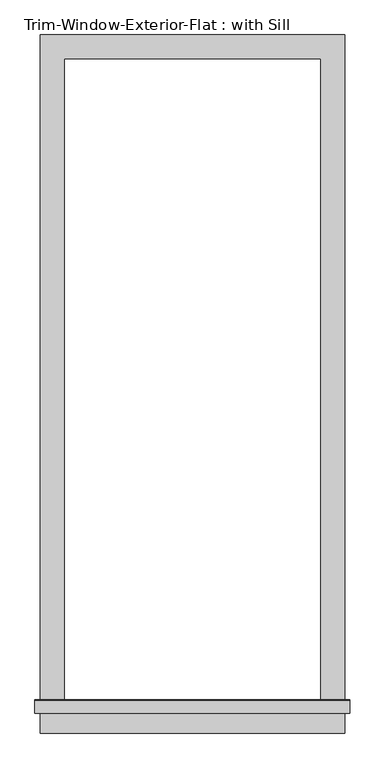
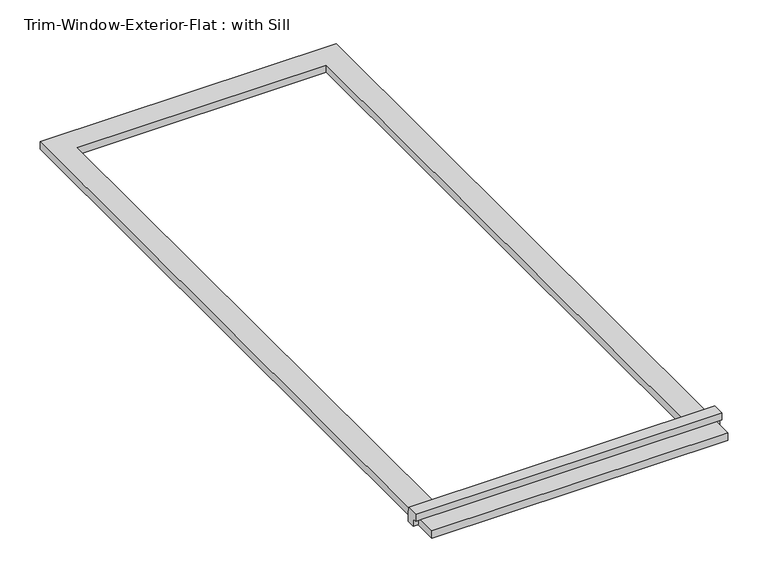
"""IFC4 building model written with IfcOpenShell, lengths in millimetres: proxy geometry, Trim-Window-Exterior-Flat : with Sill."""

from ifc_helpers import new_model, si_unit, frame, origin, origin_with_axes, place, context, project, spatial, polyline, outline, extrude, source, transform, mapped, element, save


def trim_window_exterior_flat_with_sill_4912eb0d(model_context):
    return source(origin(), model_context, "Body", "SweptSolid", [
        extrude(outline(polyline([(361.95, -1546.1823709), (361.95, -1603.3323709), (-361.95, -1603.3323709), (-361.95, -1546.1823709), (361.95, -1546.1823709)])), origin_with_axes(), (0.0, 0.0, 1.0), 19.05),
        extrude(outline(polyline([(-1555.75, 38.1), (-1526.4580645, 38.1), (-1524.0, 19.05), (-1524.0, 0.0), (-1546.1823709, 0.0), (-1546.1823709, 19.05), (-1555.75, 19.05), (-1555.75, 38.1)])), frame((-374.65, 0.0, 0.0), z_axis=(1.0, 0.0, 0.0), x_axis=(0.0, 1.0, 0.0)), (0.0, 0.0, 1.0), 749.3),
        extrude(outline(polyline([(-361.95, 57.15), (361.95, 57.15), (361.95, -1524.0), (304.8, -1524.0), (304.8, 0.0), (-304.8, 0.0), (-304.8, -1524.0), (-361.95, -1524.0), (-361.95, 57.15)])), origin_with_axes(), (0.0, 0.0, 1.0), 19.05),
    ])


if __name__ == "__main__":
    model = new_model("IFC4")
    model_context = context("Model", 3, world=origin())
    ifc_project = project(units=[si_unit("LENGTHUNIT", "METRE", prefix="MILLI")], contexts=[model_context])
    site = spatial("IfcSite", under=ifc_project)
    building = spatial("IfcBuilding", under=site)
    placement = place(None, origin())
    trim_window_exterior_flat_with_sill_shape = trim_window_exterior_flat_with_sill_4912eb0d(model_context)
    element("IfcBuildingElementProxy", 1, Name="Trim-Window-Exterior-Flat : with Sill", ObjectType="Trim-Window-Exterior-Flat : with Sill", at=placement, inside=building, context=model_context, shape_type="MappedRepresentation", body=[
        mapped(trim_window_exterior_flat_with_sill_shape, transform((0.0, 0.0, 0.0), x_axis=(1.0, 0.0, 0.0), y_axis=(0.0, 1.0, 0.0), z_axis=(0.0, 0.0, 1.0))),
    ])
    save(model, "model.ifc")

# Revit data of these elements
# Type "Trim-Window-Exterior-Flat : with Sill"
#   Trim Width = 0' - 2 1/4"
#   Trim Thickness_Picture Frame = 0' - 1 1/4"
#   Trim Thickness_with Sill = 0' - 0 3/4"
#   Sill Thickness = 0' - 1 1/4"
#   Opening Width [instance default] = 2' - 0"
#   Opening Height [instance default] = 3' - 0"
#   Default Elevation = 4' - 0"
#   Sill = yes
#   Picture Frame = no
#   Trim Material [instance default] = none
# Element 1 (IfcBuildingElementProxy, "Trim-Window-Exterior-Flat : with Sill")
#   Opening Height = 5' - 0"
#   Trim Material = Clad - White
#   Materials on its faces: "Clad - White"
# Materials
#   "Clad - White": class "Wood", colour RGB 242 242 238, transparency 0, Cost = 0
